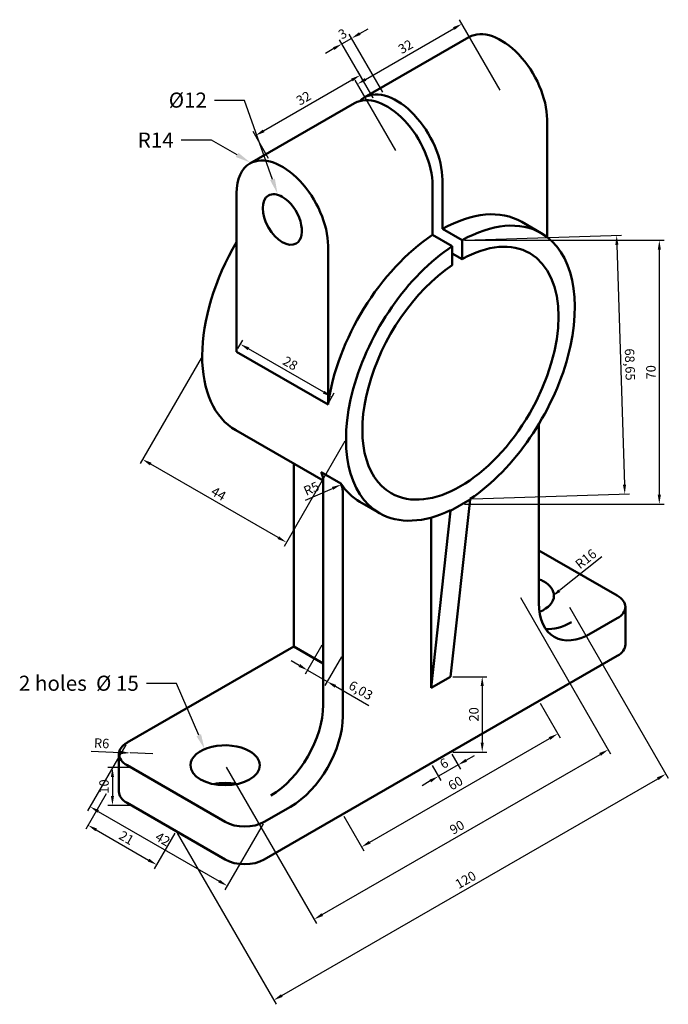
# Model space of a CAD drawing. Units: millimetres. Extents: x 2376 to 2548, y 1987 to 2248.
import ezdxf
from ezdxf import colors
from ezdxf.entities.mleader import LeaderData, LeaderLine
from ezdxf.math import Vec2, Vec3

# ---------------------------------------------------------------- set-up
doc = ezdxf.new("R2010")
doc.units = ezdxf.units.MM
doc.layers.add('M-DIMS', color=2, linetype='Continuous', lineweight=25)
doc.layers.add('M-OUTL', color=7, linetype='Continuous', lineweight=50)
doc.styles.get("Standard").update_dxf_attribs({"font": 'arial.ttf'})
doc.dimstyles.new('ISO-25', dxfattribs={"dimtxt": 2.5, "dimasz": 2.5, "dimexe": 1.25, "dimexo": 0.625, "dimtad": 1, "dimtxsty": 'Standard', "dimcen": 2.5, "dimadec": 0, "dimazin": 0, "dimtfac": 1, "dimtmove": 0, "dimatfit": 3, "dimfxl": 1, "dimarcsym": 0})

# ---------------------------------------------------------------- blocks, each defined once
blk = doc.blocks.new('*D1')
at = {"layer": 'Defpoints', "color": 0, "transparency": 16777216}
for p in [(2489.96, 2053.86), (2484.76, 2050.86), (2486.73, 2047.44)]:
    blk.add_point(p, dxfattribs=at)
at = {"layer": 'M-DIMS', "color": 0, "lineweight": -2, "transparency": 16777216}
for p, q in [((2490.27, 2053.32), (2492.56, 2049.35)), ((2494.1, 2051.69), (2496.26, 2052.94)), ((2485.07, 2050.32), (2487.36, 2046.35)), ((2491.93, 2050.44), (2486.73, 2047.44)), ((2484.57, 2046.19), (2482.4, 2044.94))]:
    blk.add_line(p, q, dxfattribs=at)
at = {"layer": 'M-DIMS', "color": 0, "transparency": 16777216}
for points in [[(2493.89, 2052.05), (2494.3, 2051.33), (2491.93, 2050.44)], [(2484.36, 2046.55), (2484.78, 2045.83), (2486.73, 2047.44)]]:
    blk.add_solid(points, dxfattribs=at)
at = {"layer": 'M-DIMS', "color": 0, "transparency": 16777216, "insert": (2488.38, 2050.58), "char_height": 2.5, "attachment_point": 5, "rotation": 30}
blk.add_mtext('6', dxfattribs=at)
blk = doc.blocks.new('*D2')
at = {"layer": 'Defpoints', "color": 0, "transparency": 16777216}
for p in [(2489.96, 2073.86), (2489.96, 2053.86), (2498.33, 2053.86)]:
    blk.add_point(p, dxfattribs=at)
at = {"layer": 'M-DIMS', "color": 0, "lineweight": -2, "transparency": 16777216}
for p, q in [((2490.58, 2073.86), (2499.58, 2073.86)), ((2498.33, 2071.36), (2498.33, 2056.36)), ((2490.58, 2053.86), (2499.58, 2053.86))]:
    blk.add_line(p, q, dxfattribs=at)
at = {"layer": 'M-DIMS', "color": 0, "transparency": 16777216}
for points in [[(2497.92, 2071.36), (2498.75, 2071.36), (2498.33, 2073.86)], [(2497.92, 2056.36), (2498.75, 2056.36), (2498.33, 2053.86)]]:
    blk.add_solid(points, dxfattribs=at)
at = {"layer": 'M-DIMS', "color": 0, "transparency": 16777216, "insert": (2496.43, 2063.86), "char_height": 2.5, "attachment_point": 5, "rotation": 90}
blk.add_mtext('20', dxfattribs=at)
blk = doc.blocks.new('*D3')
at = {"layer": 'Defpoints', "color": 0, "transparency": 16777216}
for p in [(2513.34, 2067.36), (2518.33, 2058.71), (2461.38, 2037.36)]:
    blk.add_point(p, dxfattribs=at)
at = {"layer": 'M-DIMS', "color": 0, "lineweight": -2, "transparency": 16777216}
for p, q in [((2513.65, 2066.82), (2518.95, 2057.63)), ((2468.53, 2029.96), (2516.16, 2057.46)), ((2461.69, 2036.82), (2466.99, 2027.63))]:
    blk.add_line(p, q, dxfattribs=at)
at = {"layer": 'M-DIMS', "color": 0, "transparency": 16777216}
for points in [[(2515.96, 2057.82), (2516.37, 2057.1), (2518.33, 2058.71)], [(2468.32, 2030.32), (2468.74, 2029.6), (2466.37, 2028.71)]]:
    blk.add_solid(points, dxfattribs=at)
at = {"layer": 'M-DIMS', "color": 0, "transparency": 16777216, "insert": (2491.4, 2045.36), "char_height": 2.5, "attachment_point": 5, "rotation": 30}
blk.add_mtext('60', dxfattribs=at)
blk = doc.blocks.new('*D4')
at = {"layer": 'Defpoints', "color": 0, "transparency": 16777216}
for p in [(2508.14, 2095.36), (2531.73, 2054.5), (2430.2, 2050.36)]:
    blk.add_point(p, dxfattribs=at)
at = {"layer": 'M-DIMS', "color": 0, "lineweight": -2, "transparency": 16777216}
for p, q in [((2508.45, 2094.82), (2532.36, 2053.41)), ((2455.96, 2010.75), (2529.57, 2053.25)), ((2430.51, 2049.82), (2454.42, 2008.41))]:
    blk.add_line(p, q, dxfattribs=at)
at = {"layer": 'M-DIMS', "color": 0, "transparency": 16777216}
for points in [[(2529.36, 2053.61), (2529.78, 2052.89), (2531.73, 2054.5)], [(2455.75, 2011.11), (2456.16, 2010.39), (2453.79, 2009.5)]]:
    blk.add_solid(points, dxfattribs=at)
at = {"layer": 'M-DIMS', "color": 0, "transparency": 16777216, "insert": (2491.81, 2033.64), "char_height": 2.5, "attachment_point": 5, "rotation": 30}
blk.add_mtext('90', dxfattribs=at)
blk = doc.blocks.new('*D5')
at = {"layer": 'Defpoints', "color": 0, "transparency": 16777216}
for p in [(2521.13, 2092.86), (2547, 2048.05), (2417.21, 2032.86)]:
    blk.add_point(p, dxfattribs=at)
at = {"layer": 'M-DIMS', "color": 0, "lineweight": -2, "transparency": 16777216}
for p, q in [((2521.45, 2092.32), (2547.63, 2046.96)), ((2445.25, 1989.3), (2544.84, 2046.8)), ((2417.52, 2032.32), (2443.71, 1986.96))]:
    blk.add_line(p, q, dxfattribs=at)
at = {"layer": 'M-DIMS', "color": 0, "transparency": 16777216}
for points in [[(2544.63, 2047.16), (2545.05, 2046.43), (2547, 2048.05)], [(2445.04, 1989.66), (2445.45, 1988.93), (2443.08, 1988.05)]]:
    blk.add_solid(points, dxfattribs=at)
at = {"layer": 'M-DIMS', "color": 0, "transparency": 16777216, "insert": (2494.09, 2019.69), "char_height": 2.5, "attachment_point": 5, "rotation": 30}
blk.add_mtext('120', dxfattribs=at)
blk = doc.blocks.new('*D6')
at = {"layer": 'Defpoints', "color": 0, "transparency": 16777216}
for p in [(2399.02, 2043.36), (2417.21, 2032.86), (2412.08, 2023.97)]:
    blk.add_point(p, dxfattribs=at)
at = {"layer": 'M-DIMS', "color": 0, "lineweight": -2, "transparency": 16777216}
for p, q in [((2398.71, 2042.82), (2393.27, 2033.38)), ((2396.06, 2033.22), (2409.91, 2025.22)), ((2416.9, 2032.32), (2411.45, 2022.88))]:
    blk.add_line(p, q, dxfattribs=at)
at = {"layer": 'M-DIMS', "color": 0, "transparency": 16777216}
for points in [[(2396.26, 2033.58), (2395.85, 2032.86), (2393.89, 2034.47)], [(2410.12, 2025.58), (2409.7, 2024.86), (2412.08, 2023.97)]]:
    blk.add_solid(points, dxfattribs=at)
at = {"layer": 'M-DIMS', "color": 0, "transparency": 16777216, "insert": (2403.92, 2030.85), "char_height": 2.5, "attachment_point": 5, "rotation": 330}
blk.add_mtext('21', dxfattribs=at)
blk = doc.blocks.new('*D7')
at = {"layer": 'Defpoints', "color": 0, "transparency": 16777216}
for p in [(2405.03, 2053.63), (2411.02, 2053.36)]:
    blk.add_point(p, dxfattribs=at)
at = {"layer": 'M-DIMS', "color": 0, "lineweight": -2, "transparency": 16777216}
for p, q in [((2394.76, 2054.09), (2402.53, 2053.74)), ((2411.02, 2053.36), (2405.03, 2053.63))]:
    blk.add_line(p, q, dxfattribs=at)
at = {"layer": 'M-DIMS', "color": 0, "transparency": 16777216}
blk.add_solid([(2402.55, 2054.15), (2402.51, 2053.32), (2405.03, 2053.63)], dxfattribs=at)
at = {"layer": 'M-DIMS', "color": 0, "transparency": 16777216, "insert": (2397.48, 2055.87), "char_height": 2.5, "attachment_point": 5, "rotation": 357.4305}
blk.add_mtext('R6', dxfattribs=at)
blk = doc.blocks.new('*D8')
at = {"layer": 'Defpoints', "color": 0, "transparency": 16777216}
for p in [(2529.34, 2105.07), (2516.81, 2095.11)]:
    blk.add_point(p, dxfattribs=at)
at = {"layer": 'M-DIMS', "color": 0, "lineweight": -2, "transparency": 16777216}
blk.add_line((2530, 2105.6), (2518.77, 2096.67), dxfattribs=at)
at = {"layer": 'M-DIMS', "color": 0, "transparency": 16777216}
blk.add_solid([(2518.51, 2096.99), (2519.03, 2096.34), (2516.81, 2095.11)], dxfattribs=at)
at = {"layer": 'M-DIMS', "color": 0, "transparency": 16777216, "insert": (2525.99, 2104.84), "char_height": 2.5, "attachment_point": 5, "rotation": 38.4859}
blk.add_mtext('R16', dxfattribs=at)
blk = doc.blocks.new('*D9')
at = {"layer": 'Defpoints', "color": 0, "transparency": 16777216}
for p in [(2406.24, 2049.73), (2400.35, 2039.73), (2406.24, 2039.73)]:
    blk.add_point(p, dxfattribs=at)
at = {"layer": 'M-DIMS', "color": 0, "lineweight": -2, "transparency": 16777216}
for p, q in [((2405.61, 2049.73), (2399.1, 2049.73)), ((2400.35, 2047.23), (2400.35, 2042.23)), ((2405.61, 2039.73), (2399.1, 2039.73))]:
    blk.add_line(p, q, dxfattribs=at)
at = {"layer": 'M-DIMS', "color": 0, "transparency": 16777216}
for points in [[(2399.94, 2047.23), (2400.77, 2047.23), (2400.35, 2049.73)], [(2399.94, 2042.23), (2400.77, 2042.23), (2400.35, 2039.73)]]:
    blk.add_solid(points, dxfattribs=at)
at = {"layer": 'M-DIMS', "color": 0, "transparency": 16777216, "insert": (2398.45, 2044.73), "char_height": 2.5, "attachment_point": 5, "rotation": 90}
blk.add_mtext('10', dxfattribs=at)
blk = doc.blocks.new('*D10')
at = {"layer": 'Defpoints', "color": 0, "transparency": 16777216}
for p in [(2456.16, 2082.72), (2461.38, 2079.7), (2457.25, 2072.56)]:
    blk.add_point(p, dxfattribs=at)
at = {"layer": 'M-DIMS', "color": 0, "lineweight": -2, "transparency": 16777216}
for p, q in [((2455.85, 2082.18), (2451.41, 2074.49)), ((2461.06, 2079.16), (2456.63, 2071.48)), ((2449.87, 2076.83), (2447.7, 2078.08)), ((2452.03, 2075.58), (2457.25, 2072.56)), ((2459.42, 2071.31), (2468.3, 2066.18))]:
    blk.add_line(p, q, dxfattribs=at)
at = {"layer": 'M-DIMS', "color": 0, "transparency": 16777216}
for points in [[(2450.08, 2077.19), (2449.66, 2076.46), (2452.03, 2075.58)], [(2459.63, 2071.67), (2459.21, 2070.95), (2457.25, 2072.56)]]:
    blk.add_solid(points, dxfattribs=at)
at = {"layer": 'M-DIMS', "color": 0, "transparency": 16777216, "insert": (2466.01, 2069.96), "char_height": 2.5, "attachment_point": 5, "rotation": 330}
blk.add_mtext('6,03', dxfattribs=at)
blk = doc.blocks.new('*D11')
at = {"layer": 'Defpoints', "color": 0, "transparency": 16777216}
for p in [(2460.95, 2124.81), (2456.38, 2122.79)]:
    blk.add_point(p, dxfattribs=at)
at = {"layer": 'M-DIMS', "color": 0, "lineweight": -2, "transparency": 16777216}
blk.add_line((2451.53, 2120.64), (2458.66, 2123.8), dxfattribs=at)
at = {"layer": 'M-DIMS', "color": 0, "transparency": 16777216}
blk.add_solid([(2458.49, 2124.18), (2458.83, 2123.42), (2460.95, 2124.81)], dxfattribs=at)
at = {"layer": 'M-DIMS', "color": 0, "transparency": 16777216, "insert": (2453.19, 2123.45), "char_height": 2.5, "attachment_point": 5, "rotation": 23.8798}
blk.add_mtext('R5', dxfattribs=at)
blk = doc.blocks.new('*D12')
at = {"layer": 'Defpoints', "color": 0, "transparency": 16777216}
for p in [(2492.97, 2189.59), (2492.97, 2119.59), (2545.25, 2119.59)]:
    blk.add_point(p, dxfattribs=at)
at = {"layer": 'M-DIMS', "color": 0, "lineweight": -2, "transparency": 16777216}
for p, q in [((2493.6, 2189.59), (2546.5, 2189.59)), ((2545.25, 2187.09), (2545.25, 2122.09)), ((2493.6, 2119.59), (2546.5, 2119.59))]:
    blk.add_line(p, q, dxfattribs=at)
at = {"layer": 'M-DIMS', "color": 0, "transparency": 16777216}
for points in [[(2544.84, 2187.09), (2545.67, 2187.09), (2545.25, 2189.59)], [(2544.84, 2122.09), (2545.67, 2122.09), (2545.25, 2119.59)]]:
    blk.add_solid(points, dxfattribs=at)
at = {"layer": 'M-DIMS', "color": 0, "transparency": 16777216, "insert": (2543.35, 2154.59), "char_height": 2.5, "attachment_point": 5, "rotation": 90}
blk.add_mtext('70', dxfattribs=at)
blk = doc.blocks.new('*D13')
at = {"layer": 'Defpoints', "color": 0, "transparency": 16777216}
for p in [(2424.14, 2158.86), (2462.24, 2136.86), (2408.34, 2131.49)]:
    blk.add_point(p, dxfattribs=at)
at = {"layer": 'M-DIMS', "color": 0, "lineweight": -2, "transparency": 16777216}
for p, q in [((2423.83, 2158.32), (2407.71, 2130.4)), ((2461.93, 2136.32), (2445.82, 2108.4)), ((2444.28, 2110.74), (2410.5, 2130.24))]:
    blk.add_line(p, q, dxfattribs=at)
at = {"layer": 'M-DIMS', "color": 0, "transparency": 16777216}
for points in [[(2410.71, 2130.6), (2410.29, 2129.88), (2408.34, 2131.49)], [(2444.48, 2111.1), (2444.07, 2110.38), (2446.44, 2109.49)]]:
    blk.add_solid(points, dxfattribs=at)
at = {"layer": 'M-DIMS', "color": 0, "transparency": 16777216, "insert": (2428.33, 2122.11), "char_height": 2.5, "attachment_point": 5, "rotation": 330}
blk.add_mtext('44', dxfattribs=at)
blk = doc.blocks.new('*D14')
at = {"layer": 'Defpoints', "color": 0, "transparency": 16777216}
for p in [(2433.29, 2160.4), (2434.24, 2162.06), (2457.54, 2146.4)]:
    blk.add_point(p, dxfattribs=at)
at = {"layer": 'M-DIMS', "color": 0, "lineweight": -2, "transparency": 16777216}
for p, q in [((2433.6, 2160.94), (2434.87, 2163.14)), ((2456.33, 2149.31), (2436.41, 2160.81)), ((2457.85, 2146.94), (2459.12, 2149.14))]:
    blk.add_line(p, q, dxfattribs=at)
at = {"layer": 'M-DIMS', "color": 0, "transparency": 16777216}
for points in [[(2436.62, 2161.17), (2436.2, 2160.45), (2434.24, 2162.06)], [(2456.54, 2149.67), (2456.12, 2148.95), (2458.49, 2148.06)]]:
    blk.add_solid(points, dxfattribs=at)
at = {"layer": 'M-DIMS', "color": 0, "transparency": 16777216, "insert": (2447.32, 2156.7), "char_height": 2.5, "attachment_point": 5, "rotation": 330}
blk.add_mtext('28', dxfattribs=at)
blk = doc.blocks.new('*D15')
at = {"layer": 'Defpoints', "color": 0, "transparency": 16777216}
for p in [(2465.97, 2233.36), (2469.76, 2226.79), (2442.05, 2210.79)]:
    blk.add_point(p, dxfattribs=at)
at = {"layer": 'M-DIMS', "color": 0, "lineweight": -2, "transparency": 16777216}
for p, q in [((2469.45, 2227.33), (2465.34, 2234.44)), ((2440.42, 2218.61), (2463.8, 2232.11)), ((2441.73, 2211.33), (2437.63, 2218.44))]:
    blk.add_line(p, q, dxfattribs=at)
at = {"layer": 'M-DIMS', "color": 0, "transparency": 16777216}
for points in [[(2463.59, 2232.47), (2464.01, 2231.75), (2465.97, 2233.36)], [(2440.21, 2218.97), (2440.63, 2218.25), (2438.25, 2217.36)]]:
    blk.add_solid(points, dxfattribs=at)
at = {"layer": 'M-DIMS', "color": 0, "transparency": 16777216, "insert": (2451.16, 2227.01), "char_height": 2.5, "attachment_point": 5, "rotation": 30}
blk.add_mtext('32', dxfattribs=at)
blk = doc.blocks.new('*D16')
at = {"layer": 'Defpoints', "color": 0, "transparency": 16777216}
for p in [(2463.74, 2243.18), (2472.33, 2228.3), (2469.73, 2226.8)]:
    blk.add_point(p, dxfattribs=at)
at = {"layer": 'M-DIMS', "color": 0, "lineweight": -2, "transparency": 16777216}
for p, q in [((2472.02, 2228.84), (2463.11, 2244.26)), ((2465.9, 2244.43), (2468.07, 2245.68)), ((2469.42, 2227.34), (2460.52, 2242.76)), ((2461.14, 2241.68), (2463.74, 2243.18)), ((2458.98, 2240.43), (2456.81, 2239.18))]:
    blk.add_line(p, q, dxfattribs=at)
at = {"layer": 'M-DIMS', "color": 0, "transparency": 16777216}
for points in [[(2465.69, 2244.79), (2466.11, 2244.07), (2463.74, 2243.18)], [(2458.77, 2240.79), (2459.18, 2240.07), (2461.14, 2241.68)]]:
    blk.add_solid(points, dxfattribs=at)
at = {"layer": 'M-DIMS', "color": 0, "transparency": 16777216, "insert": (2461.49, 2244.07), "char_height": 2.5, "attachment_point": 5, "rotation": 30}
blk.add_mtext('3', dxfattribs=at)
blk = doc.blocks.new('*D17')
at = {"layer": 'Defpoints', "color": 0, "transparency": 16777216}
for p in [(2492.97, 2247.02), (2503.44, 2228.9), (2475.72, 2212.9)]:
    blk.add_point(p, dxfattribs=at)
at = {"layer": 'M-DIMS', "color": 0, "lineweight": -2, "transparency": 16777216}
for p, q in [((2503.12, 2229.44), (2492.35, 2248.1)), ((2467.43, 2232.27), (2490.81, 2245.77)), ((2475.41, 2213.44), (2464.64, 2232.1))]:
    blk.add_line(p, q, dxfattribs=at)
at = {"layer": 'M-DIMS', "color": 0, "transparency": 16777216}
for points in [[(2490.6, 2246.13), (2491.02, 2245.41), (2492.97, 2247.02)], [(2467.22, 2232.63), (2467.63, 2231.91), (2465.26, 2231.02)]]:
    blk.add_solid(points, dxfattribs=at)
at = {"layer": 'M-DIMS', "color": 0, "transparency": 16777216, "insert": (2478.17, 2240.67), "char_height": 2.5, "attachment_point": 5, "rotation": 30}
blk.add_mtext('32', dxfattribs=at)
blk = doc.blocks.new('*D18')
at = {"layer": 'Defpoints', "color": 0, "transparency": 16777216}
for p in [(2404.22, 2056.36), (2440.59, 2035.36), (2430.79, 2018.38)]:
    blk.add_point(p, dxfattribs=at)
at = {"layer": 'M-DIMS', "color": 0, "lineweight": -2, "transparency": 16777216}
for p, q in [((2403.91, 2055.81), (2393.79, 2038.3)), ((2396.58, 2038.13), (2428.63, 2019.63)), ((2440.28, 2034.81), (2430.17, 2017.3))]:
    blk.add_line(p, q, dxfattribs=at)
at = {"layer": 'M-DIMS', "color": 0, "transparency": 16777216}
for points in [[(2396.79, 2038.49), (2396.37, 2037.77), (2394.42, 2039.38)], [(2428.83, 2019.99), (2428.42, 2019.27), (2430.79, 2018.38)]]:
    blk.add_solid(points, dxfattribs=at)
at = {"layer": 'M-DIMS', "color": 0, "transparency": 16777216, "insert": (2413.54, 2030.51), "char_height": 2.5, "attachment_point": 5, "rotation": 330}
blk.add_mtext('42', dxfattribs=at)
blk = doc.blocks.new('*D19')
at = {"layer": 'Defpoints', "color": 0, "transparency": 16777216}
for p in [(2492.99, 2189.6), (2495.15, 2120.99), (2536.1, 2122.28)]:
    blk.add_point(p, dxfattribs=at)
at = {"layer": 'M-DIMS', "color": 0, "lineweight": -2, "transparency": 16777216}
for p, q in [((2493.61, 2189.62), (2535.19, 2190.93)), ((2534.02, 2188.4), (2536.02, 2124.78)), ((2495.78, 2121), (2537.35, 2122.32))]:
    blk.add_line(p, q, dxfattribs=at)
at = {"layer": 'M-DIMS', "color": 0, "transparency": 16777216}
for points in [[(2534.43, 2188.41), (2533.6, 2188.38), (2533.94, 2190.89)], [(2536.44, 2124.79), (2535.61, 2124.76), (2536.1, 2122.28)]]:
    blk.add_solid(points, dxfattribs=at)
at = {"layer": 'M-DIMS', "color": 0, "transparency": 16777216, "insert": (2537.15, 2156.65), "char_height": 2.5, "attachment_point": 5, "rotation": 271.8072}
blk.add_mtext('68,65', dxfattribs=at)

msp = doc.modelspace()

# ---------------------------------------------------------------- linework, layer by layer
at = {"layer": 'M-OUTL'}
for p, q in [((2494.806, 2243.455), (2467.093, 2227.455)), ((2464.495, 2225.955), (2436.782, 2209.955)), ((2515.504, 2221.606), (2515.504, 2190.47)), ((2485.193, 2204.106), (2485.193, 2191.017)), ((2487.791, 2205.606), (2487.791, 2192.603)), ((2433.231, 2160.001), (2433.231, 2202.106)), ((2513.987, 2191.479), (2508.791, 2194.479)), ((2490.389, 2188.017), (2485.193, 2191.017)), ((2492.987, 2189.603), (2487.791, 2192.603)), ((2492.987, 2189.603), (2492.987, 2184.602)), ((2457.48, 2188.106), (2457.48, 2146.001)), ((2490.389, 2188.017), (2490.389, 2183.002)), ((2492.987, 2184.602), (2490.389, 2186.102)), ((2457.48, 2146.001), (2433.231, 2160.001)), ((2456.181, 2125.859), (2433.016, 2139.233)), ((2513.339, 2140.881), (2513.339, 2093.356)), ((2448.387, 2081.856), (2448.387, 2130.359)), ((2455.641, 2128.098), (2460.837, 2125.098)), ((2456.181, 2066.356), (2456.181, 2125.991)), ((2461.377, 2063.356), (2461.377, 2122.991)), ((2495.152, 2120.856), (2489.956, 2073.856)), ((2495.152, 2120.856), (2489.956, 2117.856)), ((2495.152, 2120.985), (2495.152, 2120.856)), ((2471.121, 2117.233), (2465.925, 2120.233)), ((2489.956, 2117.856), (2484.76, 2070.856)), ((2489.956, 2117.985), (2489.956, 2117.856)), ((2484.76, 2070.856), (2484.76, 2116.033)), ((2534.123, 2095.356), (2513.339, 2107.356)), ((2536.276, 2082.356), (2536.276, 2092.356)), ((2527.195, 2085.356), (2534.123, 2089.356)), ((2404.219, 2056.356), (2448.387, 2081.856)), ((2456.181, 2077.356), (2448.387, 2081.856)), ((2440.593, 2025.356), (2534.123, 2079.356)), ((2484.76, 2070.856), (2489.956, 2073.856)), ((2402.067, 2043.356), (2402.067, 2053.356)), ((2430.2, 2035.356), (2404.219, 2050.356)), ((2430.2, 2025.356), (2404.219, 2040.356)), ((2440.593, 2035.356), (2447.521, 2039.356))]:
    msp.add_line(p, q, dxfattribs=at)
for centre, major_axis, start_param, end_param in [((2503.379, 2228.606), (8.573, -14.849), 0.7853982, 3.1415927), ((2473.068, 2211.106), (-8.573, 14.849), 3.9269908, 6.2831853), ((2475.667, 2212.606), (-8.573, 14.849), 3.9269908, 6.2831853), ((2475.667, 2212.606), (-8.573, 14.849), 0, 0.1521088), ((2445.356, 2195.106), (8.573, -14.849), 0.7853982, 3.1415927), ((2445.356, 2195.106), (8.573, -14.849), 3.1415927, 3.9269908), ((2445.356, 2195.106), (3.674, -6.364), 3.1415927, 6.2831853), ((2445.356, 2195.106), (3.674, -6.364), 2.3561945, 3.1415927), ((2445.356, 2195.106), (3.674, -6.364), 0, 2.3561945), ((2487.358, 2157.356), (21.433, 37.123), 0, 0.771112), ((2492.554, 2154.356), (21.433, 37.123), 0, 0.771112), ((2487.358, 2157.356), (21.433, 37.123), 0.8568876, 2.1869618), ((2492.554, 2154.356), (21.433, 37.123), 4.0128104, 6.2831853), ((2454.449, 2176.356), (-21.433, -37.123), 4.7023883, 6.2831853), ((2492.554, 2154.356), (18.371, 31.82), 0, 0.7687307), ((2492.554, 2154.356), (21.433, 37.123), 0.8568876, 3.1415927), ((2492.554, 2154.356), (18.371, 31.82), 3.1415927, 6.2831853), ((2492.554, 2154.356), (18.371, 31.82), 0.8688283, 3.1415927), ((2451.85, 2123.491), (-3.062, -5.304), 2.3562328, 2.8609471), ((2487.358, 2157.356), (21.433, 37.123), 2.8616363, 3.1415927), ((2457.046, 2120.491), (-3.062, -5.304), 2.3562328, 2.8609471), ((2492.554, 2154.356), (21.433, 37.123), 3.1415927, 3.8411712), ((2508.142, 2095.356), (9.186, 0), 0.7853982, 0.9695321), ((2508.142, 2095.356), (9.186, 0), 0, 0.7853982), ((2508.142, 2095.356), (9.186, 0), 5.334505, 6.2831853), ((2528.927, 2092.356), (7.348, 0), 0, 0.7853982), ((2527.195, 2101.356), (-9.798, -16.971), 5.4977871, 6.2831853), ((2528.927, 2092.356), (7.348, 0), 5.4977871, 6.2831853), ((2521.999, 2104.356), (-9.798, -16.971), 0.2683751, 0.7853982), ((2527.195, 2101.356), (-9.798, -16.971), 0, 0.7853982), ((2528.927, 2082.356), (7.348, 0), 5.4977871, 6.2831853), ((2442.325, 2058.356), (-9.798, -16.971), 0.7853982, 2.3561945), ((2447.521, 2055.356), (-9.798, -16.971), 0.7853982, 2.3561945), ((2409.416, 2053.356), (-7.348, 0), 5.4977871, 6.2831853), ((2430.2, 2050.356), (9.186, 0), 0.7853982, 3.1415927), ((2409.416, 2053.356), (-7.348, 0), 0, 0.7853982), ((2430.2, 2050.356), (9.186, 0), 0, 0.7853982), ((2430.2, 2050.356), (9.186, 0), 3.1415927, 6.2831853), ((2430.2, 2040.356), (9.186, 0), 1.2309594, 1.9106332), ((2409.416, 2043.356), (-7.348, 0), 0, 0.7853982), ((2435.396, 2038.356), (7.348, 0), 3.9269908, 5.4977871), ((2435.396, 2028.356), (7.348, 0), 3.9269908, 5.4977871)]:
    msp.add_ellipse(centre, major_axis=major_axis, ratio=0.5773503, start_param=start_param, end_param=end_param, dxfattribs=at)

# ---------------------------------------------------------------- dimensions: what is measured, and where the dimension line sits
at = {"layer": 'M-DIMS'}
for p1, p2, distance, picture, middle in [((2469.729, 2226.8), (2472.328, 2228.3), 17.179, '*D16', (2461.488, 2244.075)), ((2475.722, 2212.9), (2503.435, 2228.9), 20.925, '*D17', (2478.165, 2240.669)), ((2442.046, 2210.793), (2469.758, 2226.793), 7.584, '*D15', (2451.159, 2227.008)), ((2492.972, 2189.595), (2492.972, 2119.595), 52.282, '*D12', (2543.352, 2154.595)), ((2457.536, 2146.4), (2433.287, 2160.4), -1.913, '*D14', (2447.319, 2156.703)), ((2462.243, 2136.856), (2424.138, 2158.856), 31.604, '*D13', (2428.326, 2122.11)), ((2430.2, 2050.356), (2508.142, 2095.356), -47.18, '*D4', (2491.811, 2033.644)), ((2417.21, 2032.856), (2521.133, 2092.856), -51.743, '*D5', (2494.092, 2019.692)), ((2456.158, 2082.717), (2461.377, 2079.704), -8.247, '*D10', (2466.007, 2069.965)), ((2489.956, 2073.856), (2489.956, 2053.856), 8.378, '*D2', (2496.433, 2063.856)), ((2461.377, 2037.356), (2513.339, 2067.356), -9.981, '*D3', (2491.398, 2045.359)), ((2489.956, 2053.856), (2484.76, 2050.856), 3.949, '*D1', (2488.382, 2050.583)), ((2406.24, 2049.734), (2406.24, 2039.734), -5.886, '*D9', (2398.453, 2044.734)), ((2399.023, 2043.356), (2417.21, 2032.856), -10.264, '*D6', (2403.925, 2030.846))]:
    dim = msp.add_aligned_dim(p1=p1, p2=p2, distance=distance, dimstyle='ISO-25', override={"dimclrd": 0, "dimclre": 0, "dimclrt": 0}, dxfattribs=at)
    dim.commit()
    dim.dimension.update_dxf_attribs({"geometry": picture, "text_midpoint": middle})
for base, p1, p2, angle, picture, middle in [((2536.102, 2122.277), (2492.987, 2189.603), (2495.152, 2120.985), 271.80723, '*D19', (2537.146, 2156.653)), ((2430.791, 2018.379), (2404.219, 2056.356), (2440.593, 2035.356), 330, '*D18', (2413.544, 2030.507))]:
    dim = msp.add_linear_dim(base=base, p1=p1, p2=p2, angle=angle, dimstyle='ISO-25', override={"dimrnd": 0}, dxfattribs=at)
    dim.commit()
    dim.dimension.update_dxf_attribs({"geometry": picture, "text_midpoint": middle})
for center, mpoint, picture, middle in [((2456.377, 2122.788), (2460.949, 2124.812), '*D11', (2453.954, 2121.715)), ((2529.339, 2105.069), (2516.814, 2095.112), '*D8', (2527.174, 2103.348))]:
    dim = msp.add_radius_dim(center=center, mpoint=mpoint, dimstyle='ISO-25', override={"dimclrd": 0, "dimclre": 0, "dimclrt": 0}, dxfattribs=at)
    dim.commit()
    dim.dimension.update_dxf_attribs({"geometry": picture, "text_midpoint": middle, "dimtype": 164})
dim = msp.add_radius_dim(center=(2411.023, 2053.356), mpoint=(2405.029, 2053.625), dimstyle='ISO-25', override={"dimclrd": 0, "dimclre": 0, "dimclrt": 0}, dxfattribs=at)
dim.commit()
dim.dimension.update_dxf_attribs({"geometry": '*D7', "text_midpoint": (2397.482, 2055.867)})

# ---------------------------------------------------------------- leaders
ml = msp.add_multileader_mtext('Standard', dxfattribs=at)
ml.set_content('Ø12', color=256)
ml.set_leader_properties()
ml.build(insert=Vec2(0, 0))
ctx = ml.context
ctx.base_point, ctx.plane_origin = Vec3(2413.348, 2226.698), Vec3(2444.094, 2201.965)
ctx.text_align_type = 2
notes = []
notes.append((ctx, [(0, (1, 1, 0), (2435.389, 2226.698), (-1, 0), 8, [(0, [(2444.094, 2201.965)], 0, [])])]))
ctx.mtext.insert, ctx.mtext.alignment, ctx.mtext.flow_direction = Vec3(2425.389, 2228.779), 3, 5
ml = msp.add_multileader_mtext('Standard', dxfattribs=at)
ml.set_content('R14', color=256)
ml.set_leader_properties()
ml.build(insert=Vec2(0, 0))
ctx = ml.context
ctx.base_point, ctx.plane_origin = Vec3(2405.042, 2216.17), Vec3(2436.838, 2210.249)
ctx.text_align_type = 2
notes.append((ctx, [(0, (1, 1, 0), (2426.583, 2216.17), (-1, 0), 8, [(0, [(2436.838, 2210.249)], 0, [])])]))
ctx.mtext.insert, ctx.mtext.alignment, ctx.mtext.flow_direction = Vec3(2416.583, 2218.17), 3, 5
ml = msp.add_multileader_mtext('Standard', dxfattribs=at)
ml.set_content('2 holes  Ø 15', color=256)
ml.set_leader_properties()
ml.build(insert=Vec2(0, 0))
ctx = ml.context
ctx.base_point, ctx.plane_origin = Vec3(2372.489, 2072.038), Vec3(2424.803, 2054.648)
ctx.text_align_type = 2
notes.append((ctx, [(0, (1, 1, 0), (2417.34, 2072.038), (-1, 0), 8, [(0, [(2424.803, 2054.648)], 0, [])])]))
ctx.mtext.insert, ctx.mtext.alignment, ctx.mtext.flow_direction = Vec3(2407.34, 2074.118), 3, 5
for ctx, leaders in notes:
    for number, flags, end, landing, length, lines in leaders:
        leader = LeaderData()
        leader.index, (leader.has_last_leader_line, leader.has_dogleg_vector, leader.attachment_direction) = number, flags
        leader.last_leader_point, leader.dogleg_vector, leader.dogleg_length = Vec3(end), Vec3(landing), length
        for number, points, colour, breaks in lines:
            line = LeaderLine()
            line.index, line.vertices, line.color, line.breaks = number, Vec3.list(points), colors.encode_raw_color(colour), breaks
            leader.lines.append(line)
        ctx.leaders.append(leader)

doc.saveas('drawing.dxf')
